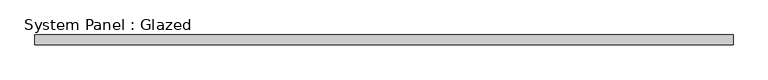
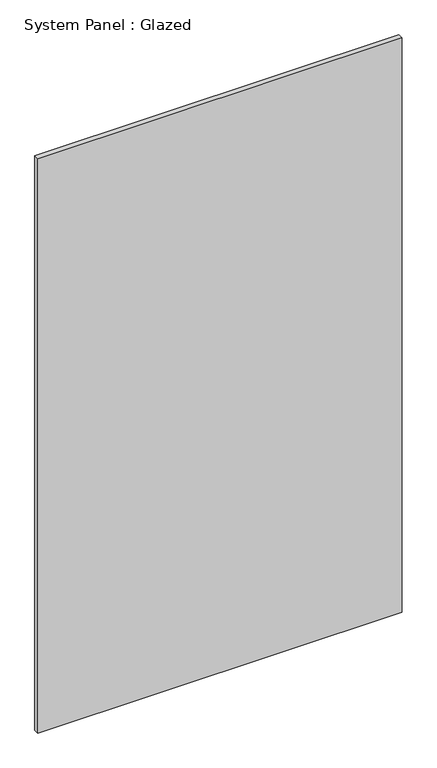
"""IFC4 building model written with IfcOpenShell, lengths in millimetres: plate geometry, System Panel : Glazed."""

from ifc_helpers import new_model, si_unit, origin, origin_with_axes, place, context, project, spatial, polyline, outline, extrude, source, transform, mapped, element, save


def system_panel_glazed_acd1c6f8(model_context):
    return source(origin(), model_context, "Body", "SweptSolid", [
        extrude(outline(polyline([(914.4, 19.05), (-914.4, 19.05), (-914.4, 44.45), (914.4, 44.45), (914.4, 19.05)])), origin_with_axes(), (0.0, 0.0, 1.0), 3048.0),
    ])


if __name__ == "__main__":
    model = new_model("IFC4")
    model_context = context("Model", 3, world=origin())
    ifc_project = project(units=[si_unit("LENGTHUNIT", "METRE", prefix="MILLI")], contexts=[model_context])
    site = spatial("IfcSite", under=ifc_project)
    building = spatial("IfcBuilding", under=site)
    placement = place(None, origin())
    system_panel_glazed_shape = system_panel_glazed_acd1c6f8(model_context)
    element("IfcPlate", 1, ObjectType="System Panel : Glazed", at=placement, inside=building, context=model_context, shape_type="MappedRepresentation", body=[
        mapped(system_panel_glazed_shape, transform((0.0, 0.0, 0.0), x_axis=(1.0, 0.0, 0.0), y_axis=(0.0, 1.0, 0.0), z_axis=(0.0, 0.0, 1.0))),
    ])
    save(model, "model.ifc")

# Revit data of these elements
# Type "System Panel : Glazed"
#   Construction Type Id = "GSP4R"
#   Analytic Construction = "1/8 in Pilkington single glazing"
#   Visual Light Transmittance = 0.9
#   Solar Heat Gain Coefficient = 0.86
#   Heat Transfer Coefficient (U) = 1.18115 BTU/(h·ft²·°F)
# Element 1 (IfcPlate, "System Panel : Glazed")
#   Materials on its faces: "Glass"
# Materials
#   "Glass": class "Glass", colour RGB 0 128 192, transparency 0.75, Description = "Soda Lime Glass", Cost = 0
